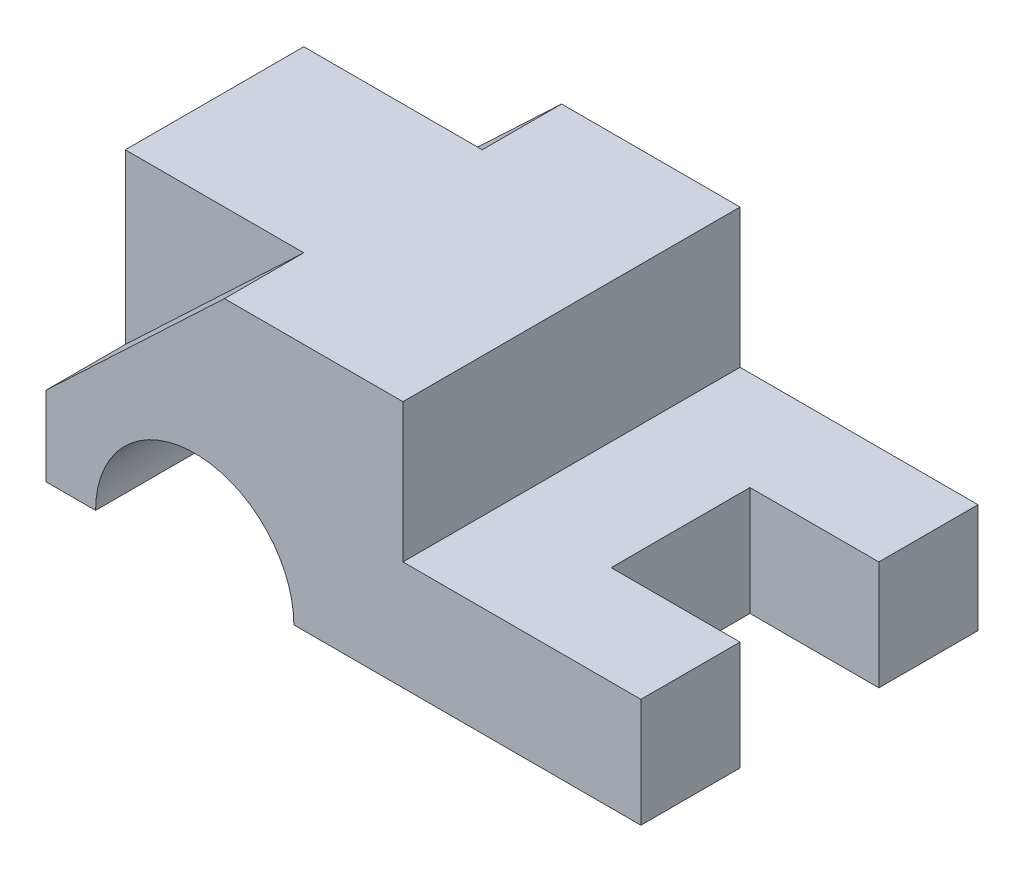
ISO-10303-21;
HEADER;
FILE_DESCRIPTION(('STEP AP214'),'2;1');
FILE_NAME('part.step','',(''),(''),'','','');
FILE_SCHEMA(('AUTOMOTIVE_DESIGN { 1 0 10303 214 1 1 1 1 }'));
ENDSEC;
DATA;
#1=APPLICATION_CONTEXT('core data for automotive mechanical design processes');
#2=APPLICATION_PROTOCOL_DEFINITION('international standard','automotive_design',2000,#1);
#3=PRODUCT_CONTEXT('',#1,'mechanical');
#4=PRODUCT('Part','Part','',(#3));
#5=PRODUCT_RELATED_PRODUCT_CATEGORY('part','',(#4));
#6=PRODUCT_DEFINITION_FORMATION('','',#4);
#7=PRODUCT_DEFINITION_CONTEXT('part definition',#1,'design');
#8=PRODUCT_DEFINITION('design','',#6,#7);
#9=PRODUCT_DEFINITION_SHAPE('','',#8);
#10=(LENGTH_UNIT() NAMED_UNIT(*) SI_UNIT(.MILLI.,.METRE.));
#11=(NAMED_UNIT(*) PLANE_ANGLE_UNIT() SI_UNIT($,.RADIAN.));
#12=(NAMED_UNIT(*) SI_UNIT($,.STERADIAN.) SOLID_ANGLE_UNIT());
#13=UNCERTAINTY_MEASURE_WITH_UNIT(LENGTH_MEASURE(1.E-05),#10,'distance_accuracy_value','');
#14=(GEOMETRIC_REPRESENTATION_CONTEXT(3) GLOBAL_UNCERTAINTY_ASSIGNED_CONTEXT((#13)) GLOBAL_UNIT_ASSIGNED_CONTEXT((#10,
#11,#12)) REPRESENTATION_CONTEXT('',''));
#15=CARTESIAN_POINT('',(0.,0.,0.));
#16=DIRECTION('',(0.,0.,1.));
#17=DIRECTION('',(1.,0.,0.));
#18=AXIS2_PLACEMENT_3D('',#15,#16,#17);
#19=CARTESIAN_POINT('',(-15.,25.,17.));
#20=DIRECTION('',(0.,-1.,0.));
#21=DIRECTION('',(0.,0.,-1.));
#22=AXIS2_PLACEMENT_3D('',#19,#20,#21);
#23=PLANE('',#22);
#24=DIRECTION('',(-1.,0.,0.));
#25=VECTOR('',#24,1.);
#26=CARTESIAN_POINT('',(-15.,25.,-17.));
#27=LINE('',#26,#25);
#28=CARTESIAN_POINT('',(21.,25.,-17.));
#29=VERTEX_POINT('',#28);
#30=CARTESIAN_POINT('',(3.,25.,-17.));
#31=VERTEX_POINT('',#30);
#32=EDGE_CURVE('E168',#29,#31,#27,.T.);
#33=ORIENTED_EDGE('',*,*,#32,.T.);
#34=DIRECTION('',(0.,0.,-1.));
#35=VECTOR('',#34,1.);
#36=CARTESIAN_POINT('',(3.,25.,-9.));
#37=LINE('',#36,#35);
#38=CARTESIAN_POINT('',(3.,25.,-9.));
#39=VERTEX_POINT('',#38);
#40=EDGE_CURVE('E53',#39,#31,#37,.T.);
#41=ORIENTED_EDGE('',*,*,#40,.F.);
#42=DIRECTION('',(1.,0.,0.));
#43=VECTOR('',#42,1.);
#44=CARTESIAN_POINT('',(0.,25.,-9.));
#45=LINE('',#44,#43);
#46=CARTESIAN_POINT('',(-15.,25.,-9.));
#47=VERTEX_POINT('',#46);
#48=EDGE_CURVE('E159',#47,#39,#45,.T.);
#49=ORIENTED_EDGE('',*,*,#48,.F.);
#50=DIRECTION('',(0.,0.,-1.));
#51=VECTOR('',#50,1.);
#52=CARTESIAN_POINT('',(-15.,25.,17.));
#53=LINE('',#52,#51);
#54=CARTESIAN_POINT('',(-15.,25.,9.00000000000001));
#55=VERTEX_POINT('',#54);
#56=EDGE_CURVE('E246',#55,#47,#53,.T.);
#57=ORIENTED_EDGE('',*,*,#56,.F.);
#58=DIRECTION('',(-1.,0.,0.));
#59=VECTOR('',#58,1.);
#60=CARTESIAN_POINT('',(-15.,25.,9.));
#61=LINE('',#60,#59);
#62=CARTESIAN_POINT('',(3.,25.,9.00000000000001));
#63=VERTEX_POINT('',#62);
#64=EDGE_CURVE('E65',#63,#55,#61,.T.);
#65=ORIENTED_EDGE('',*,*,#64,.F.);
#66=DIRECTION('',(0.,0.,-1.));
#67=VECTOR('',#66,1.);
#68=CARTESIAN_POINT('',(3.,25.,121.194124675467));
#69=LINE('',#68,#67);
#70=CARTESIAN_POINT('',(3.,25.,17.));
#71=VERTEX_POINT('',#70);
#72=EDGE_CURVE('E176',#71,#63,#69,.T.);
#73=ORIENTED_EDGE('',*,*,#72,.F.);
#74=DIRECTION('',(-1.,0.,0.));
#75=VECTOR('',#74,1.);
#76=CARTESIAN_POINT('',(-15.,25.,17.));
#77=LINE('',#76,#75);
#78=CARTESIAN_POINT('',(21.,25.,17.));
#79=VERTEX_POINT('',#78);
#80=EDGE_CURVE('E223',#79,#71,#77,.T.);
#81=ORIENTED_EDGE('',*,*,#80,.F.);
#82=DIRECTION('',(0.,0.,-1.));
#83=VECTOR('',#82,1.);
#84=CARTESIAN_POINT('',(21.,25.,17.));
#85=LINE('',#84,#83);
#86=EDGE_CURVE('E247',#79,#29,#85,.T.);
#87=ORIENTED_EDGE('',*,*,#86,.T.);
#88=EDGE_LOOP('',(#33,#41,#49,#57,#65,#73,#81,#87));
#89=FACE_BOUND('',#88,.T.);
#90=ADVANCED_FACE('F39',(#89),#23,.F.);
#91=CARTESIAN_POINT('',(45.,11.,17.));
#92=DIRECTION('',(-1.,0.,0.));
#93=DIRECTION('',(0.,0.,1.));
#94=AXIS2_PLACEMENT_3D('',#91,#92,#93);
#95=PLANE('',#94);
#96=DIRECTION('',(0.,0.,-1.));
#97=VECTOR('',#96,1.);
#98=CARTESIAN_POINT('',(45.,0.,17.));
#99=LINE('',#98,#97);
#100=CARTESIAN_POINT('',(45.,0.,17.));
#101=VERTEX_POINT('',#100);
#102=CARTESIAN_POINT('',(45.,0.,7.));
#103=VERTEX_POINT('',#102);
#104=EDGE_CURVE('E257',#101,#103,#99,.T.);
#105=ORIENTED_EDGE('',*,*,#104,.T.);
#106=DIRECTION('',(0.,1.,0.));
#107=VECTOR('',#106,1.);
#108=CARTESIAN_POINT('',(45.,-6.,7.));
#109=LINE('',#108,#107);
#110=CARTESIAN_POINT('',(45.,11.,7.));
#111=VERTEX_POINT('',#110);
#112=EDGE_CURVE('E193',#103,#111,#109,.T.);
#113=ORIENTED_EDGE('',*,*,#112,.T.);
#114=DIRECTION('',(0.,0.,-1.));
#115=VECTOR('',#114,1.);
#116=CARTESIAN_POINT('',(45.,11.,17.));
#117=LINE('',#116,#115);
#118=CARTESIAN_POINT('',(45.,11.,17.));
#119=VERTEX_POINT('',#118);
#120=EDGE_CURVE('E258',#119,#111,#117,.T.);
#121=ORIENTED_EDGE('',*,*,#120,.F.);
#122=DIRECTION('',(0.,1.,0.));
#123=VECTOR('',#122,1.);
#124=CARTESIAN_POINT('',(45.,11.,17.));
#125=LINE('',#124,#123);
#126=EDGE_CURVE('E218',#101,#119,#125,.T.);
#127=ORIENTED_EDGE('',*,*,#126,.F.);
#128=EDGE_LOOP('',(#105,#113,#121,#127));
#129=FACE_BOUND('',#128,.T.);
#130=ADVANCED_FACE('F290',(#129),#95,.F.);
#131=CARTESIAN_POINT('',(-10.,0.,17.));
#132=DIRECTION('',(0.,1.,0.));
#133=DIRECTION('',(-1.,0.,0.));
#134=AXIS2_PLACEMENT_3D('',#131,#132,#133);
#135=PLANE('',#134);
#136=DIRECTION('',(1.,0.,0.));
#137=VECTOR('',#136,1.);
#138=CARTESIAN_POINT('',(-10.,0.,-17.));
#139=LINE('',#138,#137);
#140=CARTESIAN_POINT('',(-15.,0.,-17.));
#141=VERTEX_POINT('',#140);
#142=CARTESIAN_POINT('',(-10.,0.,-17.));
#143=VERTEX_POINT('',#142);
#144=EDGE_CURVE('E209',#141,#143,#139,.T.);
#145=ORIENTED_EDGE('',*,*,#144,.T.);
#146=DIRECTION('',(0.,0.,-1.));
#147=VECTOR('',#146,1.);
#148=CARTESIAN_POINT('',(-10.,0.,17.));
#149=LINE('',#148,#147);
#150=CARTESIAN_POINT('',(-10.,0.,17.));
#151=VERTEX_POINT('',#150);
#152=EDGE_CURVE('E266',#151,#143,#149,.T.);
#153=ORIENTED_EDGE('',*,*,#152,.F.);
#154=DIRECTION('',(1.,0.,0.));
#155=VECTOR('',#154,1.);
#156=CARTESIAN_POINT('',(-10.,0.,17.));
#157=LINE('',#156,#155);
#158=CARTESIAN_POINT('',(-15.,0.,17.));
#159=VERTEX_POINT('',#158);
#160=EDGE_CURVE('E211',#159,#151,#157,.T.);
#161=ORIENTED_EDGE('',*,*,#160,.F.);
#162=DIRECTION('',(0.,0.,-1.));
#163=VECTOR('',#162,1.);
#164=CARTESIAN_POINT('',(-15.,0.,17.));
#165=LINE('',#164,#163);
#166=EDGE_CURVE('E228',#159,#141,#165,.T.);
#167=ORIENTED_EDGE('',*,*,#166,.T.);
#168=EDGE_LOOP('',(#145,#153,#161,#167));
#169=FACE_BOUND('',#168,.T.);
#170=ADVANCED_FACE('F41',(#169),#135,.F.);
#171=CARTESIAN_POINT('',(0.,0.,17.));
#172=DIRECTION('',(0.,0.,-1.));
#173=DIRECTION('',(-1.,0.,0.));
#174=AXIS2_PLACEMENT_3D('',#171,#172,#173);
#175=CYLINDRICAL_SURFACE('',#174,10.);
#176=CARTESIAN_POINT('',(0.,0.,-17.));
#177=DIRECTION('',(0.,0.,-1.));
#178=DIRECTION('',(1.,0.,0.));
#179=AXIS2_PLACEMENT_3D('',#176,#177,#178);
#180=CIRCLE('',#179,10.);
#181=CARTESIAN_POINT('',(10.,0.,-17.));
#182=VERTEX_POINT('',#181);
#183=EDGE_CURVE('E235',#143,#182,#180,.T.);
#184=ORIENTED_EDGE('',*,*,#183,.T.);
#185=DIRECTION('',(0.,0.,-1.));
#186=VECTOR('',#185,1.);
#187=CARTESIAN_POINT('',(10.,0.,17.));
#188=LINE('',#187,#186);
#189=CARTESIAN_POINT('',(10.,0.,17.));
#190=VERTEX_POINT('',#189);
#191=EDGE_CURVE('E263',#190,#182,#188,.T.);
#192=ORIENTED_EDGE('',*,*,#191,.F.);
#193=CARTESIAN_POINT('',(0.,0.,17.));
#194=DIRECTION('',(0.,0.,-1.));
#195=DIRECTION('',(1.,0.,0.));
#196=AXIS2_PLACEMENT_3D('',#193,#194,#195);
#197=CIRCLE('',#196,10.);
#198=EDGE_CURVE('E212',#151,#190,#197,.T.);
#199=ORIENTED_EDGE('',*,*,#198,.F.);
#200=ORIENTED_EDGE('',*,*,#152,.T.);
#201=EDGE_LOOP('',(#184,#192,#199,#200));
#202=FACE_BOUND('',#201,.T.);
#203=ADVANCED_FACE('F345',(#202),#175,.F.);
#204=CARTESIAN_POINT('',(45.,0.,17.));
#205=DIRECTION('',(0.,1.,0.));
#206=DIRECTION('',(-1.,0.,0.));
#207=AXIS2_PLACEMENT_3D('',#204,#205,#206);
#208=PLANE('',#207);
#209=DIRECTION('',(0.,0.,1.));
#210=VECTOR('',#209,1.);
#211=CARTESIAN_POINT('',(32.,0.,17.));
#212=LINE('',#211,#210);
#213=CARTESIAN_POINT('',(32.,0.,-7.));
#214=VERTEX_POINT('',#213);
#215=CARTESIAN_POINT('',(32.,0.,7.));
#216=VERTEX_POINT('',#215);
#217=EDGE_CURVE('E204',#214,#216,#212,.T.);
#218=ORIENTED_EDGE('',*,*,#217,.T.);
#219=DIRECTION('',(1.,0.,0.));
#220=VECTOR('',#219,1.);
#221=CARTESIAN_POINT('',(45.,0.,7.));
#222=LINE('',#221,#220);
#223=EDGE_CURVE('E210',#216,#103,#222,.T.);
#224=ORIENTED_EDGE('',*,*,#223,.T.);
#225=ORIENTED_EDGE('',*,*,#104,.F.);
#226=DIRECTION('',(1.,0.,0.));
#227=VECTOR('',#226,1.);
#228=CARTESIAN_POINT('',(45.,0.,17.));
#229=LINE('',#228,#227);
#230=EDGE_CURVE('E220',#190,#101,#229,.T.);
#231=ORIENTED_EDGE('',*,*,#230,.F.);
#232=ORIENTED_EDGE('',*,*,#191,.T.);
#233=DIRECTION('',(1.,0.,0.));
#234=VECTOR('',#233,1.);
#235=CARTESIAN_POINT('',(45.,0.,-17.));
#236=LINE('',#235,#234);
#237=CARTESIAN_POINT('',(45.,0.,-17.));
#238=VERTEX_POINT('',#237);
#239=EDGE_CURVE('E234',#182,#238,#236,.T.);
#240=ORIENTED_EDGE('',*,*,#239,.T.);
#241=CARTESIAN_POINT('',(45.,0.,-7.));
#242=VERTEX_POINT('',#241);
#243=EDGE_CURVE('E259',#242,#238,#99,.T.);
#244=ORIENTED_EDGE('',*,*,#243,.F.);
#245=DIRECTION('',(-1.,0.,0.));
#246=VECTOR('',#245,1.);
#247=CARTESIAN_POINT('',(45.,0.,-7.));
#248=LINE('',#247,#246);
#249=EDGE_CURVE('E194',#242,#214,#248,.T.);
#250=ORIENTED_EDGE('',*,*,#249,.T.);
#251=EDGE_LOOP('',(#218,#224,#225,#231,#232,#240,#244,#250));
#252=FACE_BOUND('',#251,.T.);
#253=ADVANCED_FACE('F282',(#252),#208,.F.);
#254=CARTESIAN_POINT('',(45.,11.,-7.));
#255=VERTEX_POINT('',#254);
#256=CARTESIAN_POINT('',(45.,11.,-17.));
#257=VERTEX_POINT('',#256);
#258=EDGE_CURVE('E254',#255,#257,#117,.T.);
#259=ORIENTED_EDGE('',*,*,#258,.F.);
#260=DIRECTION('',(0.,1.,0.));
#261=VECTOR('',#260,1.);
#262=CARTESIAN_POINT('',(45.,-6.,-7.));
#263=LINE('',#262,#261);
#264=EDGE_CURVE('E190',#242,#255,#263,.T.);
#265=ORIENTED_EDGE('',*,*,#264,.F.);
#266=ORIENTED_EDGE('',*,*,#243,.T.);
#267=DIRECTION('',(0.,1.,0.));
#268=VECTOR('',#267,1.);
#269=CARTESIAN_POINT('',(45.,11.,-17.));
#270=LINE('',#269,#268);
#271=EDGE_CURVE('E240',#238,#257,#270,.T.);
#272=ORIENTED_EDGE('',*,*,#271,.T.);
#273=EDGE_LOOP('',(#259,#265,#266,#272));
#274=FACE_BOUND('',#273,.T.);
#275=ADVANCED_FACE('F302',(#274),#95,.F.);
#276=CARTESIAN_POINT('',(21.,11.,17.));
#277=DIRECTION('',(0.,-1.,0.));
#278=DIRECTION('',(1.,0.,0.));
#279=AXIS2_PLACEMENT_3D('',#276,#277,#278);
#280=PLANE('',#279);
#281=ORIENTED_EDGE('',*,*,#120,.T.);
#282=DIRECTION('',(-1.,0.,0.));
#283=VECTOR('',#282,1.);
#284=CARTESIAN_POINT('',(21.,11.,7.));
#285=LINE('',#284,#283);
#286=CARTESIAN_POINT('',(32.,11.,7.));
#287=VERTEX_POINT('',#286);
#288=EDGE_CURVE('E11',#111,#287,#285,.T.);
#289=ORIENTED_EDGE('',*,*,#288,.T.);
#290=DIRECTION('',(0.,0.,-1.));
#291=VECTOR('',#290,1.);
#292=CARTESIAN_POINT('',(32.,11.,17.));
#293=LINE('',#292,#291);
#294=CARTESIAN_POINT('',(32.,11.,-7.));
#295=VERTEX_POINT('',#294);
#296=EDGE_CURVE('E50',#287,#295,#293,.T.);
#297=ORIENTED_EDGE('',*,*,#296,.T.);
#298=DIRECTION('',(1.,0.,0.));
#299=VECTOR('',#298,1.);
#300=CARTESIAN_POINT('',(21.,11.,-7.));
#301=LINE('',#300,#299);
#302=EDGE_CURVE('E267',#295,#255,#301,.T.);
#303=ORIENTED_EDGE('',*,*,#302,.T.);
#304=ORIENTED_EDGE('',*,*,#258,.T.);
#305=DIRECTION('',(-1.,0.,0.));
#306=VECTOR('',#305,1.);
#307=CARTESIAN_POINT('',(21.,11.,-17.));
#308=LINE('',#307,#306);
#309=CARTESIAN_POINT('',(21.,11.,-17.));
#310=VERTEX_POINT('',#309);
#311=EDGE_CURVE('E238',#257,#310,#308,.T.);
#312=ORIENTED_EDGE('',*,*,#311,.T.);
#313=DIRECTION('',(0.,0.,-1.));
#314=VECTOR('',#313,1.);
#315=CARTESIAN_POINT('',(21.,11.,17.));
#316=LINE('',#315,#314);
#317=CARTESIAN_POINT('',(21.,11.,17.));
#318=VERTEX_POINT('',#317);
#319=EDGE_CURVE('E252',#318,#310,#316,.T.);
#320=ORIENTED_EDGE('',*,*,#319,.F.);
#321=DIRECTION('',(-1.,0.,0.));
#322=VECTOR('',#321,1.);
#323=CARTESIAN_POINT('',(21.,11.,17.));
#324=LINE('',#323,#322);
#325=EDGE_CURVE('E222',#119,#318,#324,.T.);
#326=ORIENTED_EDGE('',*,*,#325,.F.);
#327=EDGE_LOOP('',(#281,#289,#297,#303,#304,#312,#320,#326));
#328=FACE_BOUND('',#327,.T.);
#329=ADVANCED_FACE('F272',(#328),#280,.F.);
#330=CARTESIAN_POINT('',(21.,25.,17.));
#331=DIRECTION('',(-1.,0.,0.));
#332=DIRECTION('',(0.,0.,1.));
#333=AXIS2_PLACEMENT_3D('',#330,#331,#332);
#334=PLANE('',#333);
#335=DIRECTION('',(0.,1.,0.));
#336=VECTOR('',#335,1.);
#337=CARTESIAN_POINT('',(21.,25.,-17.));
#338=LINE('',#337,#336);
#339=EDGE_CURVE('E245',#310,#29,#338,.T.);
#340=ORIENTED_EDGE('',*,*,#339,.T.);
#341=ORIENTED_EDGE('',*,*,#86,.F.);
#342=DIRECTION('',(0.,1.,0.));
#343=VECTOR('',#342,1.);
#344=CARTESIAN_POINT('',(21.,25.,17.));
#345=LINE('',#344,#343);
#346=EDGE_CURVE('E224',#318,#79,#345,.T.);
#347=ORIENTED_EDGE('',*,*,#346,.F.);
#348=ORIENTED_EDGE('',*,*,#319,.T.);
#349=EDGE_LOOP('',(#340,#341,#347,#348));
#350=FACE_BOUND('',#349,.T.);
#351=ADVANCED_FACE('F331',(#350),#334,.F.);
#352=CARTESIAN_POINT('',(-15.,0.,17.));
#353=DIRECTION('',(1.,0.,0.));
#354=DIRECTION('',(0.,0.,-1.));
#355=AXIS2_PLACEMENT_3D('',#352,#353,#354);
#356=PLANE('',#355);
#357=DIRECTION('',(0.,1.,0.));
#358=VECTOR('',#357,1.);
#359=CARTESIAN_POINT('',(-15.,0.,-9.));
#360=LINE('',#359,#358);
#361=CARTESIAN_POINT('',(-15.,8.,-9.));
#362=VERTEX_POINT('',#361);
#363=EDGE_CURVE('E157',#362,#47,#360,.T.);
#364=ORIENTED_EDGE('',*,*,#363,.F.);
#365=DIRECTION('',(0.,0.,-1.));
#366=VECTOR('',#365,1.);
#367=CARTESIAN_POINT('',(-15.,8.,-9.));
#368=LINE('',#367,#366);
#369=CARTESIAN_POINT('',(-15.,8.,-17.));
#370=VERTEX_POINT('',#369);
#371=EDGE_CURVE('E156',#362,#370,#368,.T.);
#372=ORIENTED_EDGE('',*,*,#371,.T.);
#373=DIRECTION('',(0.,-1.,0.));
#374=VECTOR('',#373,1.);
#375=CARTESIAN_POINT('',(-15.,0.,-17.));
#376=LINE('',#375,#374);
#377=EDGE_CURVE('E214',#370,#141,#376,.T.);
#378=ORIENTED_EDGE('',*,*,#377,.T.);
#379=ORIENTED_EDGE('',*,*,#166,.F.);
#380=DIRECTION('',(0.,-1.,0.));
#381=VECTOR('',#380,1.);
#382=CARTESIAN_POINT('',(-15.,0.,17.));
#383=LINE('',#382,#381);
#384=CARTESIAN_POINT('',(-15.,7.99999999999999,17.));
#385=VERTEX_POINT('',#384);
#386=EDGE_CURVE('E230',#385,#159,#383,.T.);
#387=ORIENTED_EDGE('',*,*,#386,.F.);
#388=DIRECTION('',(0.,0.,-1.));
#389=VECTOR('',#388,1.);
#390=CARTESIAN_POINT('',(-15.,7.99999999999999,121.194124675467));
#391=LINE('',#390,#389);
#392=CARTESIAN_POINT('',(-15.,7.99999999999999,9.00000000000001));
#393=VERTEX_POINT('',#392);
#394=EDGE_CURVE('E185',#385,#393,#391,.T.);
#395=ORIENTED_EDGE('',*,*,#394,.T.);
#396=DIRECTION('',(0.,-1.,0.));
#397=VECTOR('',#396,1.);
#398=CARTESIAN_POINT('',(-15.,0.,9.));
#399=LINE('',#398,#397);
#400=EDGE_CURVE('E179',#55,#393,#399,.T.);
#401=ORIENTED_EDGE('',*,*,#400,.F.);
#402=ORIENTED_EDGE('',*,*,#56,.T.);
#403=EDGE_LOOP('',(#364,#372,#378,#379,#387,#395,#401,#402));
#404=FACE_BOUND('',#403,.T.);
#405=ADVANCED_FACE('F335',(#404),#356,.F.);
#406=CARTESIAN_POINT('',(0.,0.,17.));
#407=DIRECTION('',(0.,0.,1.));
#408=DIRECTION('',(1.,0.,0.));
#409=AXIS2_PLACEMENT_3D('',#406,#407,#408);
#410=PLANE('',#409);
#411=DIRECTION('',(0.727013152549818,0.686623532963716,0.));
#412=VECTOR('',#411,1.);
#413=CARTESIAN_POINT('',(-15.,7.99999999999999,17.));
#414=LINE('',#413,#412);
#415=EDGE_CURVE('E184',#385,#71,#414,.T.);
#416=ORIENTED_EDGE('',*,*,#415,.F.);
#417=ORIENTED_EDGE('',*,*,#386,.T.);
#418=ORIENTED_EDGE('',*,*,#160,.T.);
#419=ORIENTED_EDGE('',*,*,#198,.T.);
#420=ORIENTED_EDGE('',*,*,#230,.T.);
#421=ORIENTED_EDGE('',*,*,#126,.T.);
#422=ORIENTED_EDGE('',*,*,#325,.T.);
#423=ORIENTED_EDGE('',*,*,#346,.T.);
#424=ORIENTED_EDGE('',*,*,#80,.T.);
#425=EDGE_LOOP('',(#416,#417,#418,#419,#420,#421,#422,#423,#424));
#426=FACE_BOUND('',#425,.T.);
#427=ADVANCED_FACE('F292',(#426),#410,.T.);
#428=CARTESIAN_POINT('',(0.,0.,-17.));
#429=DIRECTION('',(0.,0.,1.));
#430=DIRECTION('',(1.,0.,0.));
#431=AXIS2_PLACEMENT_3D('',#428,#429,#430);
#432=PLANE('',#431);
#433=ORIENTED_EDGE('',*,*,#377,.F.);
#434=DIRECTION('',(-0.727013152549817,-0.686623532963716,0.));
#435=VECTOR('',#434,1.);
#436=CARTESIAN_POINT('',(-11.0652528548124,11.7161500815661,-17.));
#437=LINE('',#436,#435);
#438=EDGE_CURVE('E164',#31,#370,#437,.T.);
#439=ORIENTED_EDGE('',*,*,#438,.F.);
#440=ORIENTED_EDGE('',*,*,#32,.F.);
#441=ORIENTED_EDGE('',*,*,#339,.F.);
#442=ORIENTED_EDGE('',*,*,#311,.F.);
#443=ORIENTED_EDGE('',*,*,#271,.F.);
#444=ORIENTED_EDGE('',*,*,#239,.F.);
#445=ORIENTED_EDGE('',*,*,#183,.F.);
#446=ORIENTED_EDGE('',*,*,#144,.F.);
#447=EDGE_LOOP('',(#433,#439,#440,#441,#442,#443,#444,#445,#446));
#448=FACE_BOUND('',#447,.T.);
#449=ADVANCED_FACE('F299',(#448),#432,.F.);
#450=CARTESIAN_POINT('',(32.,-6.,7.));
#451=DIRECTION('',(0.,0.,1.));
#452=DIRECTION('',(1.,0.,0.));
#453=AXIS2_PLACEMENT_3D('',#450,#451,#452);
#454=PLANE('',#453);
#455=DIRECTION('',(0.,1.,0.));
#456=VECTOR('',#455,1.);
#457=CARTESIAN_POINT('',(32.,-6.,7.));
#458=LINE('',#457,#456);
#459=EDGE_CURVE('E192',#216,#287,#458,.T.);
#460=ORIENTED_EDGE('',*,*,#459,.T.);
#461=ORIENTED_EDGE('',*,*,#288,.F.);
#462=ORIENTED_EDGE('',*,*,#112,.F.);
#463=ORIENTED_EDGE('',*,*,#223,.F.);
#464=EDGE_LOOP('',(#460,#461,#462,#463));
#465=FACE_BOUND('',#464,.T.);
#466=ADVANCED_FACE('F278',(#465),#454,.F.);
#467=CARTESIAN_POINT('',(32.,-6.,-7.));
#468=DIRECTION('',(-1.,0.,0.));
#469=DIRECTION('',(0.,-1.,0.));
#470=AXIS2_PLACEMENT_3D('',#467,#468,#469);
#471=PLANE('',#470);
#472=DIRECTION('',(0.,1.,0.));
#473=VECTOR('',#472,1.);
#474=CARTESIAN_POINT('',(32.,-6.,-7.));
#475=LINE('',#474,#473);
#476=EDGE_CURVE('E196',#214,#295,#475,.T.);
#477=ORIENTED_EDGE('',*,*,#476,.T.);
#478=ORIENTED_EDGE('',*,*,#296,.F.);
#479=ORIENTED_EDGE('',*,*,#459,.F.);
#480=ORIENTED_EDGE('',*,*,#217,.F.);
#481=EDGE_LOOP('',(#477,#478,#479,#480));
#482=FACE_BOUND('',#481,.T.);
#483=ADVANCED_FACE('F280',(#482),#471,.F.);
#484=CARTESIAN_POINT('',(45.,-6.,-7.));
#485=DIRECTION('',(0.,0.,-1.));
#486=DIRECTION('',(-1.,0.,0.));
#487=AXIS2_PLACEMENT_3D('',#484,#485,#486);
#488=PLANE('',#487);
#489=ORIENTED_EDGE('',*,*,#264,.T.);
#490=ORIENTED_EDGE('',*,*,#302,.F.);
#491=ORIENTED_EDGE('',*,*,#476,.F.);
#492=ORIENTED_EDGE('',*,*,#249,.F.);
#493=EDGE_LOOP('',(#489,#490,#491,#492));
#494=FACE_BOUND('',#493,.T.);
#495=ADVANCED_FACE('F306',(#494),#488,.F.);
#496=CARTESIAN_POINT('',(-15.,7.99999999999999,121.194124675467));
#497=DIRECTION('',(-0.686623532963716,0.727013152549818,0.));
#498=DIRECTION('',(-0.727013152549818,-0.686623532963716,0.));
#499=AXIS2_PLACEMENT_3D('',#496,#497,#498);
#500=PLANE('',#499);
#501=ORIENTED_EDGE('',*,*,#394,.F.);
#502=ORIENTED_EDGE('',*,*,#415,.T.);
#503=ORIENTED_EDGE('',*,*,#72,.T.);
#504=DIRECTION('',(0.727013152549818,0.686623532963716,0.));
#505=VECTOR('',#504,1.);
#506=CARTESIAN_POINT('',(-15.,7.99999999999999,8.99999999999999));
#507=LINE('',#506,#505);
#508=EDGE_CURVE('E178',#393,#63,#507,.T.);
#509=ORIENTED_EDGE('',*,*,#508,.F.);
#510=EDGE_LOOP('',(#501,#502,#503,#509));
#511=FACE_BOUND('',#510,.T.);
#512=ADVANCED_FACE('F309',(#511),#500,.T.);
#513=CARTESIAN_POINT('',(0.,0.,9.));
#514=DIRECTION('',(0.,0.,1.));
#515=DIRECTION('',(1.,0.,0.));
#516=AXIS2_PLACEMENT_3D('',#513,#514,#515);
#517=PLANE('',#516);
#518=ORIENTED_EDGE('',*,*,#508,.T.);
#519=ORIENTED_EDGE('',*,*,#64,.T.);
#520=ORIENTED_EDGE('',*,*,#400,.T.);
#521=EDGE_LOOP('',(#518,#519,#520));
#522=FACE_BOUND('',#521,.T.);
#523=ADVANCED_FACE('F320',(#522),#517,.T.);
#524=CARTESIAN_POINT('',(-11.0652528548124,11.7161500815661,-9.));
#525=DIRECTION('',(0.686623532963716,-0.727013152549817,0.));
#526=DIRECTION('',(0.727013152549817,0.686623532963716,0.));
#527=AXIS2_PLACEMENT_3D('',#524,#525,#526);
#528=PLANE('',#527);
#529=ORIENTED_EDGE('',*,*,#438,.T.);
#530=ORIENTED_EDGE('',*,*,#371,.F.);
#531=DIRECTION('',(-0.727013152549817,-0.686623532963716,0.));
#532=VECTOR('',#531,1.);
#533=CARTESIAN_POINT('',(-11.0652528548124,11.7161500815661,-9.));
#534=LINE('',#533,#532);
#535=EDGE_CURVE('E155',#39,#362,#534,.T.);
#536=ORIENTED_EDGE('',*,*,#535,.F.);
#537=ORIENTED_EDGE('',*,*,#40,.T.);
#538=EDGE_LOOP('',(#529,#530,#536,#537));
#539=FACE_BOUND('',#538,.T.);
#540=ADVANCED_FACE('F152',(#539),#528,.F.);
#541=CARTESIAN_POINT('',(0.,0.,-9.));
#542=DIRECTION('',(0.,0.,-1.));
#543=DIRECTION('',(-1.,0.,0.));
#544=AXIS2_PLACEMENT_3D('',#541,#542,#543);
#545=PLANE('',#544);
#546=ORIENTED_EDGE('',*,*,#48,.T.);
#547=ORIENTED_EDGE('',*,*,#535,.T.);
#548=ORIENTED_EDGE('',*,*,#363,.T.);
#549=EDGE_LOOP('',(#546,#547,#548));
#550=FACE_BOUND('',#549,.T.);
#551=ADVANCED_FACE('F162',(#550),#545,.T.);
#552=CLOSED_SHELL('',(#90,#130,#170,#203,#253,#275,#329,#351,#405,#427,#449,#466,#483,#495,#512,
#523,#540,#551));
#553=MANIFOLD_SOLID_BREP('B2',#552);
#554=ADVANCED_BREP_SHAPE_REPRESENTATION('',(#18,#553),#14);
#555=SHAPE_DEFINITION_REPRESENTATION(#9,#554);
ENDSEC;
END-ISO-10303-21;
